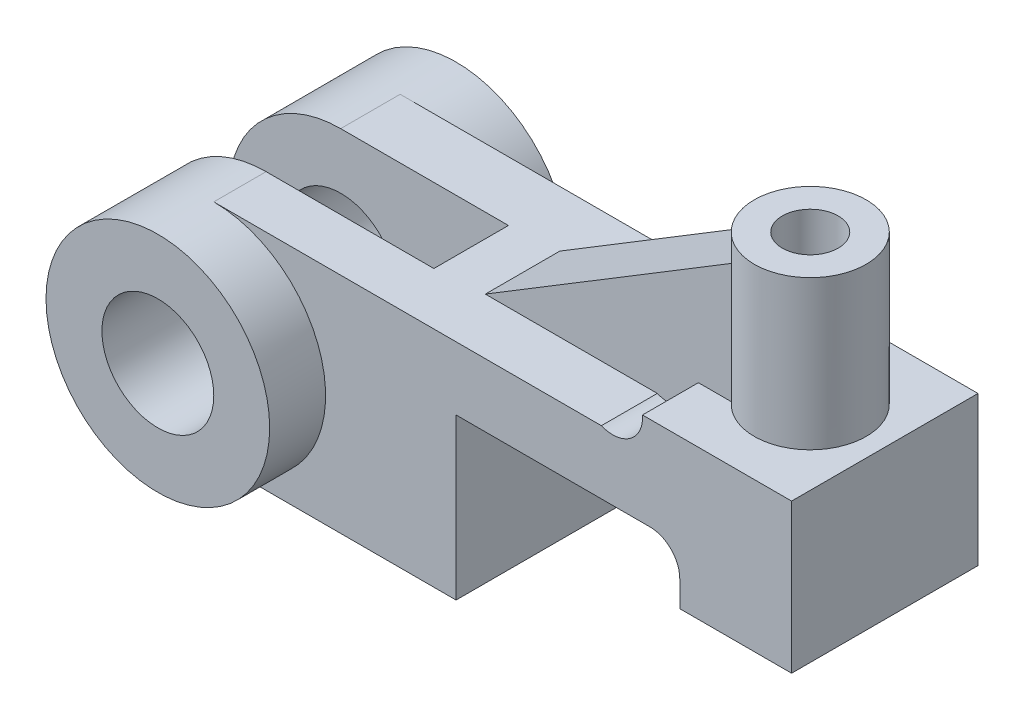
ISO-10303-21;
HEADER;
FILE_DESCRIPTION(('STEP AP214'),'2;1');
FILE_NAME('part.step','',(''),(''),'','','');
FILE_SCHEMA(('AUTOMOTIVE_DESIGN { 1 0 10303 214 1 1 1 1 }'));
ENDSEC;
DATA;
#1=APPLICATION_CONTEXT('core data for automotive mechanical design processes');
#2=APPLICATION_PROTOCOL_DEFINITION('international standard','automotive_design',2000,#1);
#3=PRODUCT_CONTEXT('',#1,'mechanical');
#4=PRODUCT('Part','Part','',(#3));
#5=PRODUCT_RELATED_PRODUCT_CATEGORY('part','',(#4));
#6=PRODUCT_DEFINITION_FORMATION('','',#4);
#7=PRODUCT_DEFINITION_CONTEXT('part definition',#1,'design');
#8=PRODUCT_DEFINITION('design','',#6,#7);
#9=PRODUCT_DEFINITION_SHAPE('','',#8);
#10=(LENGTH_UNIT() NAMED_UNIT(*) SI_UNIT(.MILLI.,.METRE.));
#11=(NAMED_UNIT(*) PLANE_ANGLE_UNIT() SI_UNIT($,.RADIAN.));
#12=(NAMED_UNIT(*) SI_UNIT($,.STERADIAN.) SOLID_ANGLE_UNIT());
#13=UNCERTAINTY_MEASURE_WITH_UNIT(LENGTH_MEASURE(1.E-05),#10,'distance_accuracy_value','');
#14=(GEOMETRIC_REPRESENTATION_CONTEXT(3) GLOBAL_UNCERTAINTY_ASSIGNED_CONTEXT((#13)) GLOBAL_UNIT_ASSIGNED_CONTEXT((#10,
#11,#12)) REPRESENTATION_CONTEXT('',''));
#15=CARTESIAN_POINT('',(0.,0.,0.));
#16=DIRECTION('',(0.,0.,1.));
#17=DIRECTION('',(1.,0.,0.));
#18=AXIS2_PLACEMENT_3D('',#15,#16,#17);
#19=CARTESIAN_POINT('',(-17.9773068022513,39.397857008049,50.));
#20=DIRECTION('',(0.,0.,-1.));
#21=DIRECTION('',(-1.,0.,0.));
#22=AXIS2_PLACEMENT_3D('',#19,#20,#21);
#23=CYLINDRICAL_SURFACE('',#22,8.);
#24=CARTESIAN_POINT('',(-17.9773068022513,39.397857008049,15.));
#25=DIRECTION('',(0.,0.,1.));
#26=DIRECTION('',(1.,0.,0.));
#27=AXIS2_PLACEMENT_3D('',#24,#25,#26);
#28=CIRCLE('',#27,8.);
#29=CARTESIAN_POINT('',(-10.,40.,15.));
#30=VERTEX_POINT('',#29);
#31=CARTESIAN_POINT('',(-21.0222553549301,32.,15.));
#32=VERTEX_POINT('',#31);
#33=EDGE_CURVE('E209',#30,#32,#28,.F.);
#34=ORIENTED_EDGE('',*,*,#33,.F.);
#35=DIRECTION('',(0.,0.,-1.));
#36=VECTOR('',#35,1.);
#37=CARTESIAN_POINT('',(-10.,40.,50.));
#38=LINE('',#37,#36);
#39=CARTESIAN_POINT('',(-10.,40.,0.));
#40=VERTEX_POINT('',#39);
#41=EDGE_CURVE('E207',#30,#40,#38,.T.);
#42=ORIENTED_EDGE('',*,*,#41,.T.);
#43=CARTESIAN_POINT('',(-17.9773068022513,39.397857008049,0.));
#44=DIRECTION('',(0.,0.,-1.));
#45=DIRECTION('',(-1.,0.,0.));
#46=AXIS2_PLACEMENT_3D('',#43,#44,#45);
#47=CIRCLE('',#46,8.);
#48=CARTESIAN_POINT('',(-21.0222553549301,32.,0.));
#49=VERTEX_POINT('',#48);
#50=EDGE_CURVE('E261',#40,#49,#47,.T.);
#51=ORIENTED_EDGE('',*,*,#50,.T.);
#52=DIRECTION('',(0.,0.,-1.));
#53=VECTOR('',#52,1.);
#54=CARTESIAN_POINT('',(-21.0222553549301,32.,50.));
#55=LINE('',#54,#53);
#56=EDGE_CURVE('E233',#32,#49,#55,.T.);
#57=ORIENTED_EDGE('',*,*,#56,.F.);
#58=EDGE_LOOP('',(#34,#42,#51,#57));
#59=FACE_BOUND('',#58,.T.);
#60=ADVANCED_FACE('F39',(#59),#23,.F.);
#61=CARTESIAN_POINT('',(-155.,32.,50.));
#62=DIRECTION('',(0.,-1.,0.));
#63=DIRECTION('',(0.,0.,-1.));
#64=AXIS2_PLACEMENT_3D('',#61,#62,#63);
#65=PLANE('',#64);
#66=CARTESIAN_POINT('',(-21.0222553549301,32.,50.));
#67=VERTEX_POINT('',#66);
#68=CARTESIAN_POINT('',(-21.0222553549301,32.,35.));
#69=VERTEX_POINT('',#68);
#70=EDGE_CURVE('E230',#67,#69,#55,.T.);
#71=ORIENTED_EDGE('',*,*,#70,.T.);
#72=DIRECTION('',(-1.,0.,0.));
#73=VECTOR('',#72,1.);
#74=CARTESIAN_POINT('',(-155.,32.,35.));
#75=LINE('',#74,#73);
#76=CARTESIAN_POINT('',(-67.1552257093281,32.,35.));
#77=VERTEX_POINT('',#76);
#78=EDGE_CURVE('E53',#69,#77,#75,.T.);
#79=ORIENTED_EDGE('',*,*,#78,.T.);
#80=DIRECTION('',(0.,0.,-1.));
#81=VECTOR('',#80,1.);
#82=CARTESIAN_POINT('',(-67.1552257093281,32.,50.));
#83=LINE('',#82,#81);
#84=CARTESIAN_POINT('',(-67.1552257093281,32.,15.));
#85=VERTEX_POINT('',#84);
#86=EDGE_CURVE('E59',#77,#85,#83,.T.);
#87=ORIENTED_EDGE('',*,*,#86,.T.);
#88=DIRECTION('',(-1.,0.,0.));
#89=VECTOR('',#88,1.);
#90=CARTESIAN_POINT('',(-155.,32.,15.));
#91=LINE('',#90,#89);
#92=EDGE_CURVE('E369',#32,#85,#91,.T.);
#93=ORIENTED_EDGE('',*,*,#92,.F.);
#94=ORIENTED_EDGE('',*,*,#56,.T.);
#95=DIRECTION('',(-1.,0.,0.));
#96=VECTOR('',#95,1.);
#97=CARTESIAN_POINT('',(-155.,32.,0.));
#98=LINE('',#97,#96);
#99=CARTESIAN_POINT('',(-125.,32.,0.));
#100=VERTEX_POINT('',#99);
#101=EDGE_CURVE('E264',#49,#100,#98,.T.);
#102=ORIENTED_EDGE('',*,*,#101,.T.);
#103=DIRECTION('',(0.,0.,1.));
#104=VECTOR('',#103,1.);
#105=CARTESIAN_POINT('',(-125.,32.,-15.));
#106=LINE('',#105,#104);
#107=CARTESIAN_POINT('',(-125.,32.,15.9553119260161));
#108=VERTEX_POINT('',#107);
#109=EDGE_CURVE('E346',#100,#108,#106,.T.);
#110=ORIENTED_EDGE('',*,*,#109,.T.);
#111=DIRECTION('',(-1.,0.,0.));
#112=VECTOR('',#111,1.);
#113=CARTESIAN_POINT('',(-155.,32.,15.9553119260161));
#114=LINE('',#113,#112);
#115=CARTESIAN_POINT('',(-80.,32.,15.9553119260161));
#116=VERTEX_POINT('',#115);
#117=EDGE_CURVE('E332',#116,#108,#114,.T.);
#118=ORIENTED_EDGE('',*,*,#117,.F.);
#119=DIRECTION('',(0.,0.,-1.));
#120=VECTOR('',#119,1.);
#121=CARTESIAN_POINT('',(-80.,32.,15.9553119260161));
#122=LINE('',#121,#120);
#123=CARTESIAN_POINT('',(-80.,32.,35.9553119260161));
#124=VERTEX_POINT('',#123);
#125=EDGE_CURVE('E336',#124,#116,#122,.T.);
#126=ORIENTED_EDGE('',*,*,#125,.F.);
#127=DIRECTION('',(1.,0.,0.));
#128=VECTOR('',#127,1.);
#129=CARTESIAN_POINT('',(-155.,32.,35.9553119260161));
#130=LINE('',#129,#128);
#131=CARTESIAN_POINT('',(-125.,32.,35.9553119260161));
#132=VERTEX_POINT('',#131);
#133=EDGE_CURVE('E331',#132,#124,#130,.T.);
#134=ORIENTED_EDGE('',*,*,#133,.F.);
#135=CARTESIAN_POINT('',(-125.,32.,50.));
#136=VERTEX_POINT('',#135);
#137=EDGE_CURVE('E352',#132,#136,#106,.T.);
#138=ORIENTED_EDGE('',*,*,#137,.T.);
#139=DIRECTION('',(-1.,0.,0.));
#140=VECTOR('',#139,1.);
#141=CARTESIAN_POINT('',(-155.,32.,50.));
#142=LINE('',#141,#140);
#143=EDGE_CURVE('E293',#67,#136,#142,.T.);
#144=ORIENTED_EDGE('',*,*,#143,.F.);
#145=EDGE_LOOP('',(#71,#79,#87,#93,#94,#102,#110,#118,#126,#134,#138,#144));
#146=FACE_BOUND('',#145,.T.);
#147=ADVANCED_FACE('F406',(#146),#65,.F.);
#148=CARTESIAN_POINT('',(-155.,-28.,35.9553119260161));
#149=DIRECTION('',(0.,0.,1.));
#150=DIRECTION('',(1.,0.,0.));
#151=AXIS2_PLACEMENT_3D('',#148,#149,#150);
#152=PLANE('',#151);
#153=CARTESIAN_POINT('',(-125.,1.99999999999999,35.9553119260161));
#154=DIRECTION('',(0.,0.,1.));
#155=DIRECTION('',(1.,0.,0.));
#156=AXIS2_PLACEMENT_3D('',#153,#154,#155);
#157=CIRCLE('',#156,15.);
#158=CARTESIAN_POINT('',(-110.,1.99999999999999,35.9553119260161));
#159=VERTEX_POINT('',#158);
#160=EDGE_CURVE('E377',#159,#159,#157,.T.);
#161=ORIENTED_EDGE('',*,*,#160,.T.);
#162=EDGE_LOOP('',(#161));
#163=FACE_BOUND('',#162,.T.);
#164=DIRECTION('',(0.,1.,0.));
#165=VECTOR('',#164,1.);
#166=CARTESIAN_POINT('',(-155.,-28.,35.9553119260161));
#167=LINE('',#166,#165);
#168=CARTESIAN_POINT('',(-155.,-28.,35.9553119260161));
#169=VERTEX_POINT('',#168);
#170=CARTESIAN_POINT('',(-155.,1.99999999999999,35.9553119260161));
#171=VERTEX_POINT('',#170);
#172=EDGE_CURVE('E329',#169,#171,#167,.T.);
#173=ORIENTED_EDGE('',*,*,#172,.T.);
#174=CARTESIAN_POINT('',(-125.,1.99999999999955,35.9553119260161));
#175=DIRECTION('',(0.,0.,1.));
#176=DIRECTION('',(1.,0.,0.));
#177=AXIS2_PLACEMENT_3D('',#174,#175,#176);
#178=CIRCLE('',#177,30.0000000000004);
#179=EDGE_CURVE('E342',#171,#132,#178,.F.);
#180=ORIENTED_EDGE('',*,*,#179,.T.);
#181=ORIENTED_EDGE('',*,*,#133,.T.);
#182=DIRECTION('',(0.,1.,0.));
#183=VECTOR('',#182,1.);
#184=CARTESIAN_POINT('',(-80.,-28.,35.9553119260161));
#185=LINE('',#184,#183);
#186=CARTESIAN_POINT('',(-80.,-28.,35.9553119260161));
#187=VERTEX_POINT('',#186);
#188=EDGE_CURVE('E322',#187,#124,#185,.T.);
#189=ORIENTED_EDGE('',*,*,#188,.F.);
#190=DIRECTION('',(1.,0.,0.));
#191=VECTOR('',#190,1.);
#192=CARTESIAN_POINT('',(-155.,-28.,35.9553119260161));
#193=LINE('',#192,#191);
#194=EDGE_CURVE('E323',#169,#187,#193,.T.);
#195=ORIENTED_EDGE('',*,*,#194,.F.);
#196=EDGE_LOOP('',(#173,#180,#181,#189,#195));
#197=FACE_BOUND('',#196,.T.);
#198=ADVANCED_FACE('F416',(#163,#197),#152,.F.);
#199=CARTESIAN_POINT('',(-155.,-28.,15.9553119260161));
#200=DIRECTION('',(0.,0.,-1.));
#201=DIRECTION('',(-1.,0.,0.));
#202=AXIS2_PLACEMENT_3D('',#199,#200,#201);
#203=PLANE('',#202);
#204=CARTESIAN_POINT('',(-125.,1.99999999999999,15.9553119260161));
#205=DIRECTION('',(0.,0.,-1.));
#206=DIRECTION('',(-1.,0.,0.));
#207=AXIS2_PLACEMENT_3D('',#204,#205,#206);
#208=CIRCLE('',#207,15.);
#209=CARTESIAN_POINT('',(-140.,1.99999999999999,15.9553119260161));
#210=VERTEX_POINT('',#209);
#211=EDGE_CURVE('E384',#210,#210,#208,.T.);
#212=ORIENTED_EDGE('',*,*,#211,.T.);
#213=EDGE_LOOP('',(#212));
#214=FACE_BOUND('',#213,.T.);
#215=CARTESIAN_POINT('',(-125.,1.99999999999955,15.9553119260161));
#216=DIRECTION('',(0.,0.,-1.));
#217=DIRECTION('',(-1.,0.,0.));
#218=AXIS2_PLACEMENT_3D('',#215,#216,#217);
#219=CIRCLE('',#218,30.0000000000004);
#220=CARTESIAN_POINT('',(-155.,1.99999999999955,15.9553119260161));
#221=VERTEX_POINT('',#220);
#222=EDGE_CURVE('E200',#108,#221,#219,.F.);
#223=ORIENTED_EDGE('',*,*,#222,.T.);
#224=DIRECTION('',(0.,1.,0.));
#225=VECTOR('',#224,1.);
#226=CARTESIAN_POINT('',(-155.,-28.,15.9553119260161));
#227=LINE('',#226,#225);
#228=CARTESIAN_POINT('',(-155.,-28.,15.9553119260161));
#229=VERTEX_POINT('',#228);
#230=EDGE_CURVE('E321',#229,#221,#227,.T.);
#231=ORIENTED_EDGE('',*,*,#230,.F.);
#232=DIRECTION('',(-1.,0.,0.));
#233=VECTOR('',#232,1.);
#234=CARTESIAN_POINT('',(-155.,-28.,15.9553119260161));
#235=LINE('',#234,#233);
#236=CARTESIAN_POINT('',(-80.,-28.,15.9553119260161));
#237=VERTEX_POINT('',#236);
#238=EDGE_CURVE('E341',#237,#229,#235,.T.);
#239=ORIENTED_EDGE('',*,*,#238,.F.);
#240=DIRECTION('',(0.,1.,0.));
#241=VECTOR('',#240,1.);
#242=CARTESIAN_POINT('',(-80.,-28.,15.9553119260161));
#243=LINE('',#242,#241);
#244=EDGE_CURVE('E325',#237,#116,#243,.T.);
#245=ORIENTED_EDGE('',*,*,#244,.T.);
#246=ORIENTED_EDGE('',*,*,#117,.T.);
#247=EDGE_LOOP('',(#223,#231,#239,#245,#246));
#248=FACE_BOUND('',#247,.T.);
#249=ADVANCED_FACE('F390',(#214,#248),#203,.F.);
#250=CARTESIAN_POINT('',(-155.,-28.,50.));
#251=DIRECTION('',(1.,0.,0.));
#252=DIRECTION('',(0.,0.,-1.));
#253=AXIS2_PLACEMENT_3D('',#250,#251,#252);
#254=PLANE('',#253);
#255=DIRECTION('',(0.,-1.,0.));
#256=VECTOR('',#255,1.);
#257=CARTESIAN_POINT('',(-155.,-28.,50.));
#258=LINE('',#257,#256);
#259=CARTESIAN_POINT('',(-155.,1.99999999999999,50.));
#260=VERTEX_POINT('',#259);
#261=CARTESIAN_POINT('',(-155.,-28.,50.));
#262=VERTEX_POINT('',#261);
#263=EDGE_CURVE('E288',#260,#262,#258,.T.);
#264=ORIENTED_EDGE('',*,*,#263,.F.);
#265=DIRECTION('',(0.,0.,1.));
#266=VECTOR('',#265,1.);
#267=CARTESIAN_POINT('',(-155.,1.99999999999999,-15.));
#268=LINE('',#267,#266);
#269=EDGE_CURVE('E354',#171,#260,#268,.T.);
#270=ORIENTED_EDGE('',*,*,#269,.F.);
#271=ORIENTED_EDGE('',*,*,#172,.F.);
#272=DIRECTION('',(0.,0.,-1.));
#273=VECTOR('',#272,1.);
#274=CARTESIAN_POINT('',(-155.,-28.,50.));
#275=LINE('',#274,#273);
#276=EDGE_CURVE('E235',#262,#169,#275,.T.);
#277=ORIENTED_EDGE('',*,*,#276,.F.);
#278=EDGE_LOOP('',(#264,#270,#271,#277));
#279=FACE_BOUND('',#278,.T.);
#280=ADVANCED_FACE('F427',(#279),#254,.F.);
#281=CARTESIAN_POINT('',(-8.,7.,0.));
#282=DIRECTION('',(0.,0.,1.));
#283=DIRECTION('',(1.,0.,0.));
#284=AXIS2_PLACEMENT_3D('',#281,#282,#283);
#285=PLANE('',#284);
#286=CARTESIAN_POINT('',(-125.,1.99999999999999,0.));
#287=DIRECTION('',(0.,0.,-1.));
#288=DIRECTION('',(-1.,0.,0.));
#289=AXIS2_PLACEMENT_3D('',#286,#287,#288);
#290=CIRCLE('',#289,30.);
#291=CARTESIAN_POINT('',(-125.,-28.,0.));
#292=VERTEX_POINT('',#291);
#293=EDGE_CURVE('E217',#100,#292,#290,.T.);
#294=ORIENTED_EDGE('',*,*,#293,.F.);
#295=ORIENTED_EDGE('',*,*,#101,.F.);
#296=ORIENTED_EDGE('',*,*,#50,.F.);
#297=DIRECTION('',(-1.,0.,0.));
#298=VECTOR('',#297,1.);
#299=CARTESIAN_POINT('',(30.,40.,0.));
#300=LINE('',#299,#298);
#301=CARTESIAN_POINT('',(30.,40.,0.));
#302=VERTEX_POINT('',#301);
#303=EDGE_CURVE('E270',#302,#40,#300,.T.);
#304=ORIENTED_EDGE('',*,*,#303,.F.);
#305=DIRECTION('',(0.,1.,0.));
#306=VECTOR('',#305,1.);
#307=CARTESIAN_POINT('',(30.,0.,0.));
#308=LINE('',#307,#306);
#309=CARTESIAN_POINT('',(30.,0.,0.));
#310=VERTEX_POINT('',#309);
#311=EDGE_CURVE('E267',#310,#302,#308,.T.);
#312=ORIENTED_EDGE('',*,*,#311,.F.);
#313=DIRECTION('',(1.,0.,0.));
#314=VECTOR('',#313,1.);
#315=CARTESIAN_POINT('',(0.,0.,0.));
#316=LINE('',#315,#314);
#317=CARTESIAN_POINT('',(0.,0.,0.));
#318=VERTEX_POINT('',#317);
#319=EDGE_CURVE('E271',#318,#310,#316,.T.);
#320=ORIENTED_EDGE('',*,*,#319,.F.);
#321=DIRECTION('',(0.,-1.,0.));
#322=VECTOR('',#321,1.);
#323=CARTESIAN_POINT('',(0.,0.,0.));
#324=LINE('',#323,#322);
#325=CARTESIAN_POINT('',(0.,6.99999999999994,0.));
#326=VERTEX_POINT('',#325);
#327=EDGE_CURVE('E277',#326,#318,#324,.T.);
#328=ORIENTED_EDGE('',*,*,#327,.F.);
#329=CARTESIAN_POINT('',(-8.,7.,0.));
#330=DIRECTION('',(0.,0.,-1.));
#331=DIRECTION('',(1.,0.,0.));
#332=AXIS2_PLACEMENT_3D('',#329,#330,#331);
#333=CIRCLE('',#332,8.);
#334=CARTESIAN_POINT('',(-8.00000000000006,15.,0.));
#335=VERTEX_POINT('',#334);
#336=EDGE_CURVE('E244',#335,#326,#333,.T.);
#337=ORIENTED_EDGE('',*,*,#336,.F.);
#338=DIRECTION('',(1.,0.,0.));
#339=VECTOR('',#338,1.);
#340=CARTESIAN_POINT('',(-8.00000000000006,15.,0.));
#341=LINE('',#340,#339);
#342=CARTESIAN_POINT('',(-60.,15.,0.));
#343=VERTEX_POINT('',#342);
#344=EDGE_CURVE('E248',#343,#335,#341,.T.);
#345=ORIENTED_EDGE('',*,*,#344,.F.);
#346=DIRECTION('',(0.,1.,0.));
#347=VECTOR('',#346,1.);
#348=CARTESIAN_POINT('',(-60.,15.,0.));
#349=LINE('',#348,#347);
#350=CARTESIAN_POINT('',(-60.,-28.,0.));
#351=VERTEX_POINT('',#350);
#352=EDGE_CURVE('E255',#351,#343,#349,.T.);
#353=ORIENTED_EDGE('',*,*,#352,.F.);
#354=DIRECTION('',(1.,0.,0.));
#355=VECTOR('',#354,1.);
#356=CARTESIAN_POINT('',(-60.,-28.,0.));
#357=LINE('',#356,#355);
#358=EDGE_CURVE('E259',#292,#351,#357,.T.);
#359=ORIENTED_EDGE('',*,*,#358,.F.);
#360=EDGE_LOOP('',(#294,#295,#296,#304,#312,#320,#328,#337,#345,#353,#359));
#361=FACE_BOUND('',#360,.T.);
#362=ADVANCED_FACE('F466',(#361),#285,.F.);
#363=CARTESIAN_POINT('',(-8.,7.,50.));
#364=DIRECTION('',(0.,0.,1.));
#365=DIRECTION('',(1.,0.,0.));
#366=AXIS2_PLACEMENT_3D('',#363,#364,#365);
#367=PLANE('',#366);
#368=CARTESIAN_POINT('',(-125.,1.99999999999999,50.));
#369=DIRECTION('',(0.,0.,1.));
#370=DIRECTION('',(1.,0.,0.));
#371=AXIS2_PLACEMENT_3D('',#368,#369,#370);
#372=CIRCLE('',#371,30.);
#373=CARTESIAN_POINT('',(-125.,-28.,50.));
#374=VERTEX_POINT('',#373);
#375=EDGE_CURVE('E302',#260,#374,#372,.T.);
#376=ORIENTED_EDGE('',*,*,#375,.F.);
#377=ORIENTED_EDGE('',*,*,#263,.T.);
#378=DIRECTION('',(1.,0.,0.));
#379=VECTOR('',#378,1.);
#380=CARTESIAN_POINT('',(-60.,-28.,50.));
#381=LINE('',#380,#379);
#382=EDGE_CURVE('E281',#262,#374,#381,.T.);
#383=ORIENTED_EDGE('',*,*,#382,.T.);
#384=EDGE_LOOP('',(#376,#377,#383));
#385=FACE_BOUND('',#384,.T.);
#386=ADVANCED_FACE('F471',(#385),#367,.T.);
#387=CARTESIAN_POINT('',(0.,0.,50.));
#388=DIRECTION('',(1.,0.,0.));
#389=DIRECTION('',(0.,0.,-1.));
#390=AXIS2_PLACEMENT_3D('',#387,#388,#389);
#391=PLANE('',#390);
#392=DIRECTION('',(0.,0.,-1.));
#393=VECTOR('',#392,1.);
#394=CARTESIAN_POINT('',(0.,6.99999999999994,50.));
#395=LINE('',#394,#393);
#396=CARTESIAN_POINT('',(0.,6.99999999999994,50.));
#397=VERTEX_POINT('',#396);
#398=EDGE_CURVE('E245',#397,#326,#395,.T.);
#399=ORIENTED_EDGE('',*,*,#398,.T.);
#400=ORIENTED_EDGE('',*,*,#327,.T.);
#401=DIRECTION('',(0.,0.,-1.));
#402=VECTOR('',#401,1.);
#403=CARTESIAN_POINT('',(0.,0.,50.));
#404=LINE('',#403,#402);
#405=CARTESIAN_POINT('',(0.,0.,50.));
#406=VERTEX_POINT('',#405);
#407=EDGE_CURVE('E220',#406,#318,#404,.T.);
#408=ORIENTED_EDGE('',*,*,#407,.F.);
#409=DIRECTION('',(0.,-1.,0.));
#410=VECTOR('',#409,1.);
#411=CARTESIAN_POINT('',(0.,0.,50.));
#412=LINE('',#411,#410);
#413=EDGE_CURVE('E247',#397,#406,#412,.T.);
#414=ORIENTED_EDGE('',*,*,#413,.F.);
#415=EDGE_LOOP('',(#399,#400,#408,#414));
#416=FACE_BOUND('',#415,.T.);
#417=ADVANCED_FACE('F41',(#416),#391,.F.);
#418=CARTESIAN_POINT('',(0.,0.,50.));
#419=DIRECTION('',(0.,1.,0.));
#420=DIRECTION('',(0.,0.,1.));
#421=AXIS2_PLACEMENT_3D('',#418,#419,#420);
#422=PLANE('',#421);
#423=ORIENTED_EDGE('',*,*,#407,.T.);
#424=ORIENTED_EDGE('',*,*,#319,.T.);
#425=DIRECTION('',(0.,0.,-1.));
#426=VECTOR('',#425,1.);
#427=CARTESIAN_POINT('',(30.,0.,50.));
#428=LINE('',#427,#426);
#429=CARTESIAN_POINT('',(30.,0.,50.));
#430=VERTEX_POINT('',#429);
#431=EDGE_CURVE('E221',#430,#310,#428,.T.);
#432=ORIENTED_EDGE('',*,*,#431,.F.);
#433=DIRECTION('',(1.,0.,0.));
#434=VECTOR('',#433,1.);
#435=CARTESIAN_POINT('',(0.,0.,50.));
#436=LINE('',#435,#434);
#437=EDGE_CURVE('E297',#406,#430,#436,.T.);
#438=ORIENTED_EDGE('',*,*,#437,.F.);
#439=EDGE_LOOP('',(#423,#424,#432,#438));
#440=FACE_BOUND('',#439,.T.);
#441=ADVANCED_FACE('F695',(#440),#422,.F.);
#442=CARTESIAN_POINT('',(30.,0.,50.));
#443=DIRECTION('',(-1.,0.,0.));
#444=DIRECTION('',(0.,0.,1.));
#445=AXIS2_PLACEMENT_3D('',#442,#443,#444);
#446=PLANE('',#445);
#447=ORIENTED_EDGE('',*,*,#431,.T.);
#448=ORIENTED_EDGE('',*,*,#311,.T.);
#449=DIRECTION('',(0.,0.,-1.));
#450=VECTOR('',#449,1.);
#451=CARTESIAN_POINT('',(30.,40.,50.));
#452=LINE('',#451,#450);
#453=CARTESIAN_POINT('',(30.,40.,50.));
#454=VERTEX_POINT('',#453);
#455=EDGE_CURVE('E223',#454,#302,#452,.T.);
#456=ORIENTED_EDGE('',*,*,#455,.F.);
#457=DIRECTION('',(0.,1.,0.));
#458=VECTOR('',#457,1.);
#459=CARTESIAN_POINT('',(30.,0.,50.));
#460=LINE('',#459,#458);
#461=EDGE_CURVE('E296',#430,#454,#460,.T.);
#462=ORIENTED_EDGE('',*,*,#461,.F.);
#463=EDGE_LOOP('',(#447,#448,#456,#462));
#464=FACE_BOUND('',#463,.T.);
#465=ADVANCED_FACE('F431',(#464),#446,.F.);
#466=CARTESIAN_POINT('',(30.,40.,50.));
#467=DIRECTION('',(0.,-1.,0.));
#468=DIRECTION('',(0.,0.,-1.));
#469=AXIS2_PLACEMENT_3D('',#466,#467,#468);
#470=PLANE('',#469);
#471=ORIENTED_EDGE('',*,*,#455,.T.);
#472=ORIENTED_EDGE('',*,*,#303,.T.);
#473=ORIENTED_EDGE('',*,*,#41,.F.);
#474=DIRECTION('',(-1.,0.,0.));
#475=VECTOR('',#474,1.);
#476=CARTESIAN_POINT('',(30.,40.,15.));
#477=LINE('',#476,#475);
#478=CARTESIAN_POINT('',(-1.18033988749895,40.,15.));
#479=VERTEX_POINT('',#478);
#480=EDGE_CURVE('E205',#479,#30,#477,.T.);
#481=ORIENTED_EDGE('',*,*,#480,.F.);
#482=CARTESIAN_POINT('',(9.99999999999999,40.,25.));
#483=DIRECTION('',(0.,-1.,0.));
#484=DIRECTION('',(0.,0.,-1.));
#485=AXIS2_PLACEMENT_3D('',#482,#483,#484);
#486=CIRCLE('',#485,15.);
#487=CARTESIAN_POINT('',(-1.18033988749895,40.,35.));
#488=VERTEX_POINT('',#487);
#489=EDGE_CURVE('E192',#488,#479,#486,.F.);
#490=ORIENTED_EDGE('',*,*,#489,.F.);
#491=DIRECTION('',(-1.,0.,0.));
#492=VECTOR('',#491,1.);
#493=CARTESIAN_POINT('',(30.,40.,35.));
#494=LINE('',#493,#492);
#495=CARTESIAN_POINT('',(-10.,40.,35.));
#496=VERTEX_POINT('',#495);
#497=EDGE_CURVE('E368',#488,#496,#494,.T.);
#498=ORIENTED_EDGE('',*,*,#497,.T.);
#499=CARTESIAN_POINT('',(-10.,40.,50.));
#500=VERTEX_POINT('',#499);
#501=EDGE_CURVE('E228',#500,#496,#38,.T.);
#502=ORIENTED_EDGE('',*,*,#501,.F.);
#503=DIRECTION('',(-1.,0.,0.));
#504=VECTOR('',#503,1.);
#505=CARTESIAN_POINT('',(30.,40.,50.));
#506=LINE('',#505,#504);
#507=EDGE_CURVE('E298',#454,#500,#506,.T.);
#508=ORIENTED_EDGE('',*,*,#507,.F.);
#509=EDGE_LOOP('',(#471,#472,#473,#481,#490,#498,#502,#508));
#510=FACE_BOUND('',#509,.T.);
#511=ADVANCED_FACE('F203',(#510),#470,.F.);
#512=ORIENTED_EDGE('',*,*,#501,.T.);
#513=CARTESIAN_POINT('',(-17.9773068022513,39.397857008049,35.));
#514=DIRECTION('',(0.,0.,1.));
#515=DIRECTION('',(1.,0.,0.));
#516=AXIS2_PLACEMENT_3D('',#513,#514,#515);
#517=CIRCLE('',#516,8.);
#518=EDGE_CURVE('E366',#496,#69,#517,.F.);
#519=ORIENTED_EDGE('',*,*,#518,.T.);
#520=ORIENTED_EDGE('',*,*,#70,.F.);
#521=CARTESIAN_POINT('',(-17.9773068022513,39.397857008049,50.));
#522=DIRECTION('',(0.,0.,-1.));
#523=DIRECTION('',(-1.,0.,0.));
#524=AXIS2_PLACEMENT_3D('',#521,#522,#523);
#525=CIRCLE('',#524,8.);
#526=EDGE_CURVE('E295',#500,#67,#525,.T.);
#527=ORIENTED_EDGE('',*,*,#526,.F.);
#528=EDGE_LOOP('',(#512,#519,#520,#527));
#529=FACE_BOUND('',#528,.T.);
#530=ADVANCED_FACE('F414',(#529),#23,.F.);
#531=ORIENTED_EDGE('',*,*,#230,.T.);
#532=CARTESIAN_POINT('',(-155.,1.99999999999999,0.));
#533=VERTEX_POINT('',#532);
#534=EDGE_CURVE('E355',#533,#221,#268,.T.);
#535=ORIENTED_EDGE('',*,*,#534,.F.);
#536=DIRECTION('',(0.,-1.,0.));
#537=VECTOR('',#536,1.);
#538=CARTESIAN_POINT('',(-155.,-28.,0.));
#539=LINE('',#538,#537);
#540=CARTESIAN_POINT('',(-155.,-28.,0.));
#541=VERTEX_POINT('',#540);
#542=EDGE_CURVE('E256',#533,#541,#539,.T.);
#543=ORIENTED_EDGE('',*,*,#542,.T.);
#544=EDGE_CURVE('E232',#229,#541,#275,.T.);
#545=ORIENTED_EDGE('',*,*,#544,.F.);
#546=EDGE_LOOP('',(#531,#535,#543,#545));
#547=FACE_BOUND('',#546,.T.);
#548=ADVANCED_FACE('F423',(#547),#254,.F.);
#549=CARTESIAN_POINT('',(-60.,-28.,50.));
#550=DIRECTION('',(0.,1.,0.));
#551=DIRECTION('',(0.,0.,1.));
#552=AXIS2_PLACEMENT_3D('',#549,#550,#551);
#553=PLANE('',#552);
#554=DIRECTION('',(0.,0.,-1.));
#555=VECTOR('',#554,1.);
#556=CARTESIAN_POINT('',(-80.,-28.,15.9553119260161));
#557=LINE('',#556,#555);
#558=EDGE_CURVE('E333',#187,#237,#557,.T.);
#559=ORIENTED_EDGE('',*,*,#558,.T.);
#560=ORIENTED_EDGE('',*,*,#238,.T.);
#561=ORIENTED_EDGE('',*,*,#544,.T.);
#562=EDGE_CURVE('E253',#541,#292,#357,.T.);
#563=ORIENTED_EDGE('',*,*,#562,.T.);
#564=ORIENTED_EDGE('',*,*,#358,.T.);
#565=DIRECTION('',(0.,0.,-1.));
#566=VECTOR('',#565,1.);
#567=CARTESIAN_POINT('',(-60.,-28.,50.));
#568=LINE('',#567,#566);
#569=CARTESIAN_POINT('',(-60.,-28.,50.));
#570=VERTEX_POINT('',#569);
#571=EDGE_CURVE('E236',#570,#351,#568,.T.);
#572=ORIENTED_EDGE('',*,*,#571,.F.);
#573=EDGE_CURVE('E290',#374,#570,#381,.T.);
#574=ORIENTED_EDGE('',*,*,#573,.F.);
#575=ORIENTED_EDGE('',*,*,#382,.F.);
#576=ORIENTED_EDGE('',*,*,#276,.T.);
#577=ORIENTED_EDGE('',*,*,#194,.T.);
#578=EDGE_LOOP('',(#559,#560,#561,#563,#564,#572,#574,#575,#576,#577));
#579=FACE_BOUND('',#578,.T.);
#580=ADVANCED_FACE('F430',(#579),#553,.F.);
#581=CARTESIAN_POINT('',(-60.,15.,50.));
#582=DIRECTION('',(-1.,0.,0.));
#583=DIRECTION('',(0.,0.,1.));
#584=AXIS2_PLACEMENT_3D('',#581,#582,#583);
#585=PLANE('',#584);
#586=ORIENTED_EDGE('',*,*,#571,.T.);
#587=ORIENTED_EDGE('',*,*,#352,.T.);
#588=DIRECTION('',(0.,0.,-1.));
#589=VECTOR('',#588,1.);
#590=CARTESIAN_POINT('',(-60.,15.,50.));
#591=LINE('',#590,#589);
#592=CARTESIAN_POINT('',(-60.,15.,50.));
#593=VERTEX_POINT('',#592);
#594=EDGE_CURVE('E238',#593,#343,#591,.T.);
#595=ORIENTED_EDGE('',*,*,#594,.F.);
#596=DIRECTION('',(0.,1.,0.));
#597=VECTOR('',#596,1.);
#598=CARTESIAN_POINT('',(-60.,15.,50.));
#599=LINE('',#598,#597);
#600=EDGE_CURVE('E282',#570,#593,#599,.T.);
#601=ORIENTED_EDGE('',*,*,#600,.F.);
#602=EDGE_LOOP('',(#586,#587,#595,#601));
#603=FACE_BOUND('',#602,.T.);
#604=ADVANCED_FACE('F481',(#603),#585,.F.);
#605=CARTESIAN_POINT('',(-8.00000000000006,15.,50.));
#606=DIRECTION('',(0.,1.,0.));
#607=DIRECTION('',(0.,0.,1.));
#608=AXIS2_PLACEMENT_3D('',#605,#606,#607);
#609=PLANE('',#608);
#610=ORIENTED_EDGE('',*,*,#594,.T.);
#611=ORIENTED_EDGE('',*,*,#344,.T.);
#612=DIRECTION('',(0.,0.,-1.));
#613=VECTOR('',#612,1.);
#614=CARTESIAN_POINT('',(-8.00000000000006,15.,50.));
#615=LINE('',#614,#613);
#616=CARTESIAN_POINT('',(-8.00000000000006,15.,50.));
#617=VERTEX_POINT('',#616);
#618=EDGE_CURVE('E239',#617,#335,#615,.T.);
#619=ORIENTED_EDGE('',*,*,#618,.F.);
#620=DIRECTION('',(1.,0.,0.));
#621=VECTOR('',#620,1.);
#622=CARTESIAN_POINT('',(-8.00000000000006,15.,50.));
#623=LINE('',#622,#621);
#624=EDGE_CURVE('E283',#593,#617,#623,.T.);
#625=ORIENTED_EDGE('',*,*,#624,.F.);
#626=EDGE_LOOP('',(#610,#611,#619,#625));
#627=FACE_BOUND('',#626,.T.);
#628=ADVANCED_FACE('F488',(#627),#609,.F.);
#629=CARTESIAN_POINT('',(-8.,7.,50.));
#630=DIRECTION('',(0.,0.,-1.));
#631=DIRECTION('',(-1.,0.,0.));
#632=AXIS2_PLACEMENT_3D('',#629,#630,#631);
#633=CYLINDRICAL_SURFACE('',#632,8.);
#634=ORIENTED_EDGE('',*,*,#618,.T.);
#635=ORIENTED_EDGE('',*,*,#336,.T.);
#636=ORIENTED_EDGE('',*,*,#398,.F.);
#637=CARTESIAN_POINT('',(-8.,7.,50.));
#638=DIRECTION('',(0.,0.,-1.));
#639=DIRECTION('',(1.,0.,0.));
#640=AXIS2_PLACEMENT_3D('',#637,#638,#639);
#641=CIRCLE('',#640,8.);
#642=EDGE_CURVE('E242',#617,#397,#641,.T.);
#643=ORIENTED_EDGE('',*,*,#642,.F.);
#644=EDGE_LOOP('',(#634,#635,#636,#643));
#645=FACE_BOUND('',#644,.T.);
#646=ADVANCED_FACE('F489',(#645),#633,.F.);
#647=EDGE_CURVE('E224',#374,#136,#372,.T.);
#648=ORIENTED_EDGE('',*,*,#647,.F.);
#649=ORIENTED_EDGE('',*,*,#573,.T.);
#650=ORIENTED_EDGE('',*,*,#600,.T.);
#651=ORIENTED_EDGE('',*,*,#624,.T.);
#652=ORIENTED_EDGE('',*,*,#642,.T.);
#653=ORIENTED_EDGE('',*,*,#413,.T.);
#654=ORIENTED_EDGE('',*,*,#437,.T.);
#655=ORIENTED_EDGE('',*,*,#461,.T.);
#656=ORIENTED_EDGE('',*,*,#507,.T.);
#657=ORIENTED_EDGE('',*,*,#526,.T.);
#658=ORIENTED_EDGE('',*,*,#143,.T.);
#659=EDGE_LOOP('',(#648,#649,#650,#651,#652,#653,#654,#655,#656,#657,#658));
#660=FACE_BOUND('',#659,.T.);
#661=ADVANCED_FACE('F491',(#660),#367,.T.);
#662=EDGE_CURVE('E310',#292,#533,#290,.T.);
#663=ORIENTED_EDGE('',*,*,#662,.F.);
#664=ORIENTED_EDGE('',*,*,#562,.F.);
#665=ORIENTED_EDGE('',*,*,#542,.F.);
#666=EDGE_LOOP('',(#663,#664,#665));
#667=FACE_BOUND('',#666,.T.);
#668=ADVANCED_FACE('F479',(#667),#285,.F.);
#669=CARTESIAN_POINT('',(-125.,1.99999999999999,65.));
#670=DIRECTION('',(0.,0.,1.));
#671=DIRECTION('',(1.,0.,0.));
#672=AXIS2_PLACEMENT_3D('',#669,#670,#671);
#673=PLANE('',#672);
#674=CARTESIAN_POINT('',(-125.,1.99999999999999,65.));
#675=DIRECTION('',(0.,0.,1.));
#676=DIRECTION('',(1.,0.,0.));
#677=AXIS2_PLACEMENT_3D('',#674,#675,#676);
#678=CIRCLE('',#677,30.);
#679=CARTESIAN_POINT('',(-95.,1.99999999999999,65.));
#680=VERTEX_POINT('',#679);
#681=EDGE_CURVE('E276',#680,#680,#678,.T.);
#682=ORIENTED_EDGE('',*,*,#681,.T.);
#683=EDGE_LOOP('',(#682));
#684=FACE_BOUND('',#683,.T.);
#685=CARTESIAN_POINT('',(-125.,1.99999999999999,65.));
#686=DIRECTION('',(0.,0.,1.));
#687=DIRECTION('',(1.,0.,0.));
#688=AXIS2_PLACEMENT_3D('',#685,#686,#687);
#689=CIRCLE('',#688,15.);
#690=CARTESIAN_POINT('',(-110.,1.99999999999999,65.));
#691=VERTEX_POINT('',#690);
#692=EDGE_CURVE('E309',#691,#691,#689,.T.);
#693=ORIENTED_EDGE('',*,*,#692,.F.);
#694=EDGE_LOOP('',(#693));
#695=FACE_BOUND('',#694,.T.);
#696=ADVANCED_FACE('F500',(#684,#695),#673,.T.);
#697=CARTESIAN_POINT('',(-125.,1.99999999999999,65.));
#698=DIRECTION('',(0.,0.,-1.));
#699=DIRECTION('',(-1.,0.,0.));
#700=AXIS2_PLACEMENT_3D('',#697,#698,#699);
#701=CYLINDRICAL_SURFACE('',#700,30.);
#702=ORIENTED_EDGE('',*,*,#681,.F.);
#703=EDGE_LOOP('',(#702));
#704=FACE_BOUND('',#703,.T.);
#705=ORIENTED_EDGE('',*,*,#647,.T.);
#706=ORIENTED_EDGE('',*,*,#137,.F.);
#707=ORIENTED_EDGE('',*,*,#179,.F.);
#708=ORIENTED_EDGE('',*,*,#269,.T.);
#709=ORIENTED_EDGE('',*,*,#375,.T.);
#710=EDGE_LOOP('',(#705,#706,#707,#708,#709));
#711=FACE_BOUND('',#710,.T.);
#712=ADVANCED_FACE('F505',(#704,#711),#701,.T.);
#713=CARTESIAN_POINT('',(-125.,1.99999999999999,65.));
#714=DIRECTION('',(0.,0.,-1.));
#715=DIRECTION('',(-1.,0.,0.));
#716=AXIS2_PLACEMENT_3D('',#713,#714,#715);
#717=CYLINDRICAL_SURFACE('',#716,15.);
#718=ORIENTED_EDGE('',*,*,#692,.T.);
#719=EDGE_LOOP('',(#718));
#720=FACE_BOUND('',#719,.T.);
#721=ORIENTED_EDGE('',*,*,#160,.F.);
#722=EDGE_LOOP('',(#721));
#723=FACE_BOUND('',#722,.T.);
#724=ADVANCED_FACE('F504',(#720,#723),#717,.F.);
#725=CARTESIAN_POINT('',(-125.,1.99999999999999,-15.));
#726=DIRECTION('',(0.,0.,-1.));
#727=DIRECTION('',(-1.,0.,0.));
#728=AXIS2_PLACEMENT_3D('',#725,#726,#727);
#729=PLANE('',#728);
#730=CARTESIAN_POINT('',(-125.,1.99999999999999,-15.));
#731=DIRECTION('',(0.,0.,-1.));
#732=DIRECTION('',(-1.,0.,0.));
#733=AXIS2_PLACEMENT_3D('',#730,#731,#732);
#734=CIRCLE('',#733,30.);
#735=CARTESIAN_POINT('',(-155.,1.99999999999999,-15.));
#736=VERTEX_POINT('',#735);
#737=EDGE_CURVE('E312',#736,#736,#734,.T.);
#738=ORIENTED_EDGE('',*,*,#737,.T.);
#739=EDGE_LOOP('',(#738));
#740=FACE_BOUND('',#739,.T.);
#741=CARTESIAN_POINT('',(-125.,1.99999999999999,-15.));
#742=DIRECTION('',(0.,0.,-1.));
#743=DIRECTION('',(-1.,0.,0.));
#744=AXIS2_PLACEMENT_3D('',#741,#742,#743);
#745=CIRCLE('',#744,15.);
#746=CARTESIAN_POINT('',(-140.,1.99999999999999,-15.));
#747=VERTEX_POINT('',#746);
#748=EDGE_CURVE('E319',#747,#747,#745,.T.);
#749=ORIENTED_EDGE('',*,*,#748,.F.);
#750=EDGE_LOOP('',(#749));
#751=FACE_BOUND('',#750,.T.);
#752=ADVANCED_FACE('F404',(#740,#751),#729,.T.);
#753=CARTESIAN_POINT('',(-125.,1.99999999999999,-15.));
#754=DIRECTION('',(0.,0.,1.));
#755=DIRECTION('',(1.,0.,0.));
#756=AXIS2_PLACEMENT_3D('',#753,#754,#755);
#757=CYLINDRICAL_SURFACE('',#756,30.);
#758=ORIENTED_EDGE('',*,*,#662,.T.);
#759=ORIENTED_EDGE('',*,*,#534,.T.);
#760=ORIENTED_EDGE('',*,*,#222,.F.);
#761=ORIENTED_EDGE('',*,*,#109,.F.);
#762=ORIENTED_EDGE('',*,*,#293,.T.);
#763=EDGE_LOOP('',(#758,#759,#760,#761,#762));
#764=FACE_BOUND('',#763,.T.);
#765=ORIENTED_EDGE('',*,*,#737,.F.);
#766=EDGE_LOOP('',(#765));
#767=FACE_BOUND('',#766,.T.);
#768=ADVANCED_FACE('F392',(#764,#767),#757,.T.);
#769=CARTESIAN_POINT('',(-125.,1.99999999999999,-15.));
#770=DIRECTION('',(0.,0.,1.));
#771=DIRECTION('',(1.,0.,0.));
#772=AXIS2_PLACEMENT_3D('',#769,#770,#771);
#773=CYLINDRICAL_SURFACE('',#772,15.);
#774=ORIENTED_EDGE('',*,*,#748,.T.);
#775=EDGE_LOOP('',(#774));
#776=FACE_BOUND('',#775,.T.);
#777=ORIENTED_EDGE('',*,*,#211,.F.);
#778=EDGE_LOOP('',(#777));
#779=FACE_BOUND('',#778,.T.);
#780=ADVANCED_FACE('F388',(#776,#779),#773,.F.);
#781=CARTESIAN_POINT('',(-80.,-28.,15.9553119260161));
#782=DIRECTION('',(1.,0.,0.));
#783=DIRECTION('',(0.,0.,-1.));
#784=AXIS2_PLACEMENT_3D('',#781,#782,#783);
#785=PLANE('',#784);
#786=ORIENTED_EDGE('',*,*,#125,.T.);
#787=ORIENTED_EDGE('',*,*,#244,.F.);
#788=ORIENTED_EDGE('',*,*,#558,.F.);
#789=ORIENTED_EDGE('',*,*,#188,.T.);
#790=EDGE_LOOP('',(#786,#787,#788,#789));
#791=FACE_BOUND('',#790,.T.);
#792=ADVANCED_FACE('F394',(#791),#785,.F.);
#793=CARTESIAN_POINT('',(9.99999999999999,80.,25.));
#794=DIRECTION('',(0.,1.,0.));
#795=DIRECTION('',(0.,0.,1.));
#796=AXIS2_PLACEMENT_3D('',#793,#794,#795);
#797=PLANE('',#796);
#798=CARTESIAN_POINT('',(9.99999999999999,80.,25.));
#799=DIRECTION('',(0.,1.,0.));
#800=DIRECTION('',(0.,0.,1.));
#801=AXIS2_PLACEMENT_3D('',#798,#799,#800);
#802=CIRCLE('',#801,7.5);
#803=CARTESIAN_POINT('',(9.99999999999999,80.,32.5));
#804=VERTEX_POINT('',#803);
#805=EDGE_CURVE('E360',#804,#804,#802,.T.);
#806=ORIENTED_EDGE('',*,*,#805,.F.);
#807=EDGE_LOOP('',(#806));
#808=FACE_BOUND('',#807,.T.);
#809=CARTESIAN_POINT('',(9.99999999999999,80.,25.));
#810=DIRECTION('',(0.,1.,0.));
#811=DIRECTION('',(0.,0.,1.));
#812=AXIS2_PLACEMENT_3D('',#809,#810,#811);
#813=CIRCLE('',#812,15.);
#814=CARTESIAN_POINT('',(9.99999999999999,80.,40.));
#815=VERTEX_POINT('',#814);
#816=EDGE_CURVE('E353',#815,#815,#813,.T.);
#817=ORIENTED_EDGE('',*,*,#816,.T.);
#818=EDGE_LOOP('',(#817));
#819=FACE_BOUND('',#818,.T.);
#820=ADVANCED_FACE('F397',(#808,#819),#797,.T.);
#821=CARTESIAN_POINT('',(9.99999999999999,80.,25.));
#822=DIRECTION('',(0.,-1.,0.));
#823=DIRECTION('',(0.,0.,-1.));
#824=AXIS2_PLACEMENT_3D('',#821,#822,#823);
#825=CYLINDRICAL_SURFACE('',#824,15.);
#826=ORIENTED_EDGE('',*,*,#816,.F.);
#827=EDGE_LOOP('',(#826));
#828=FACE_BOUND('',#827,.T.);
#829=ORIENTED_EDGE('',*,*,#489,.T.);
#830=DIRECTION('',(0.,-1.,0.));
#831=VECTOR('',#830,1.);
#832=CARTESIAN_POINT('',(-1.18033988749895,80.,15.));
#833=LINE('',#832,#831);
#834=CARTESIAN_POINT('',(-1.18033988749895,72.1244752132156,15.));
#835=VERTEX_POINT('',#834);
#836=EDGE_CURVE('E50',#835,#479,#833,.T.);
#837=ORIENTED_EDGE('',*,*,#836,.F.);
#838=CARTESIAN_POINT('',(9.99999999999999,78.9241121523802,25.));
#839=DIRECTION('',(-0.519624208779797,0.854394921362463,0.));
#840=DIRECTION('',(-0.854394921362463,-0.519624208779797,0.));
#841=AXIS2_PLACEMENT_3D('',#838,#839,#840);
#842=ELLIPSE('',#841,17.5562841315585,15.);
#843=CARTESIAN_POINT('',(-1.18033988749894,72.1244752132156,35.));
#844=VERTEX_POINT('',#843);
#845=EDGE_CURVE('E372',#835,#844,#842,.T.);
#846=ORIENTED_EDGE('',*,*,#845,.T.);
#847=DIRECTION('',(0.,-1.,0.));
#848=VECTOR('',#847,1.);
#849=CARTESIAN_POINT('',(-1.18033988749895,80.,35.));
#850=LINE('',#849,#848);
#851=EDGE_CURVE('E11',#844,#488,#850,.T.);
#852=ORIENTED_EDGE('',*,*,#851,.T.);
#853=EDGE_LOOP('',(#829,#837,#846,#852));
#854=FACE_BOUND('',#853,.T.);
#855=ADVANCED_FACE('F194',(#828,#854),#825,.T.);
#856=CARTESIAN_POINT('',(9.99999999999999,80.,25.));
#857=DIRECTION('',(0.,-1.,0.));
#858=DIRECTION('',(0.,0.,-1.));
#859=AXIS2_PLACEMENT_3D('',#856,#857,#858);
#860=CYLINDRICAL_SURFACE('',#859,7.5);
#861=ORIENTED_EDGE('',*,*,#805,.T.);
#862=EDGE_LOOP('',(#861));
#863=FACE_BOUND('',#862,.T.);
#864=CARTESIAN_POINT('',(9.99999999999999,40.,25.));
#865=DIRECTION('',(0.,1.,0.));
#866=DIRECTION('',(0.,0.,1.));
#867=AXIS2_PLACEMENT_3D('',#864,#865,#866);
#868=CIRCLE('',#867,7.5);
#869=CARTESIAN_POINT('',(9.99999999999999,40.,32.5));
#870=VERTEX_POINT('',#869);
#871=EDGE_CURVE('E359',#870,#870,#868,.T.);
#872=ORIENTED_EDGE('',*,*,#871,.F.);
#873=EDGE_LOOP('',(#872));
#874=FACE_BOUND('',#873,.T.);
#875=ADVANCED_FACE('F455',(#863,#874),#860,.F.);
#876=ORIENTED_EDGE('',*,*,#871,.T.);
#877=EDGE_LOOP('',(#876));
#878=FACE_BOUND('',#877,.T.);
#879=ADVANCED_FACE('F435',(#878),#470,.F.);
#880=CARTESIAN_POINT('',(-62.5,26.,35.));
#881=DIRECTION('',(0.,0.,1.));
#882=DIRECTION('',(1.,0.,0.));
#883=AXIS2_PLACEMENT_3D('',#880,#881,#882);
#884=PLANE('',#883);
#885=ORIENTED_EDGE('',*,*,#78,.F.);
#886=ORIENTED_EDGE('',*,*,#518,.F.);
#887=ORIENTED_EDGE('',*,*,#497,.F.);
#888=ORIENTED_EDGE('',*,*,#851,.F.);
#889=DIRECTION('',(-0.854394921362463,-0.519624208779797,0.));
#890=VECTOR('',#889,1.);
#891=CARTESIAN_POINT('',(-5.,69.8014419014058,35.));
#892=LINE('',#891,#890);
#893=EDGE_CURVE('E376',#844,#77,#892,.T.);
#894=ORIENTED_EDGE('',*,*,#893,.T.);
#895=EDGE_LOOP('',(#885,#886,#887,#888,#894));
#896=FACE_BOUND('',#895,.T.);
#897=ADVANCED_FACE('F437',(#896),#884,.T.);
#898=CARTESIAN_POINT('',(-62.5,26.,15.));
#899=DIRECTION('',(0.,0.,1.));
#900=DIRECTION('',(1.,0.,0.));
#901=AXIS2_PLACEMENT_3D('',#898,#899,#900);
#902=PLANE('',#901);
#903=ORIENTED_EDGE('',*,*,#33,.T.);
#904=ORIENTED_EDGE('',*,*,#92,.T.);
#905=DIRECTION('',(-0.854394921362463,-0.519624208779797,0.));
#906=VECTOR('',#905,1.);
#907=CARTESIAN_POINT('',(-5.,69.8014419014058,15.));
#908=LINE('',#907,#906);
#909=EDGE_CURVE('E211',#835,#85,#908,.T.);
#910=ORIENTED_EDGE('',*,*,#909,.F.);
#911=ORIENTED_EDGE('',*,*,#836,.T.);
#912=ORIENTED_EDGE('',*,*,#480,.T.);
#913=EDGE_LOOP('',(#903,#904,#910,#911,#912));
#914=FACE_BOUND('',#913,.T.);
#915=ADVANCED_FACE('F215',(#914),#902,.F.);
#916=CARTESIAN_POINT('',(-5.,69.8014419014058,25.));
#917=DIRECTION('',(-0.519624208779797,0.854394921362463,0.));
#918=DIRECTION('',(-0.854394921362463,-0.519624208779797,0.));
#919=AXIS2_PLACEMENT_3D('',#916,#917,#918);
#920=PLANE('',#919);
#921=ORIENTED_EDGE('',*,*,#86,.F.);
#922=ORIENTED_EDGE('',*,*,#893,.F.);
#923=ORIENTED_EDGE('',*,*,#845,.F.);
#924=ORIENTED_EDGE('',*,*,#909,.T.);
#925=EDGE_LOOP('',(#921,#922,#923,#924));
#926=FACE_BOUND('',#925,.T.);
#927=ADVANCED_FACE('F445',(#926),#920,.T.);
#928=CLOSED_SHELL('',(#60,#147,#198,#249,#280,#362,#386,#417,#441,#465,#511,#530,#548,#580,#604,
#628,#646,#661,#668,#696,#712,#724,#752,#768,#780,#792,#820,#855,#875,#879,#897,#915,#927));
#929=MANIFOLD_SOLID_BREP('B2',#928);
#930=ADVANCED_BREP_SHAPE_REPRESENTATION('',(#18,#929),#14);
#931=SHAPE_DEFINITION_REPRESENTATION(#9,#930);
ENDSEC;
END-ISO-10303-21;
